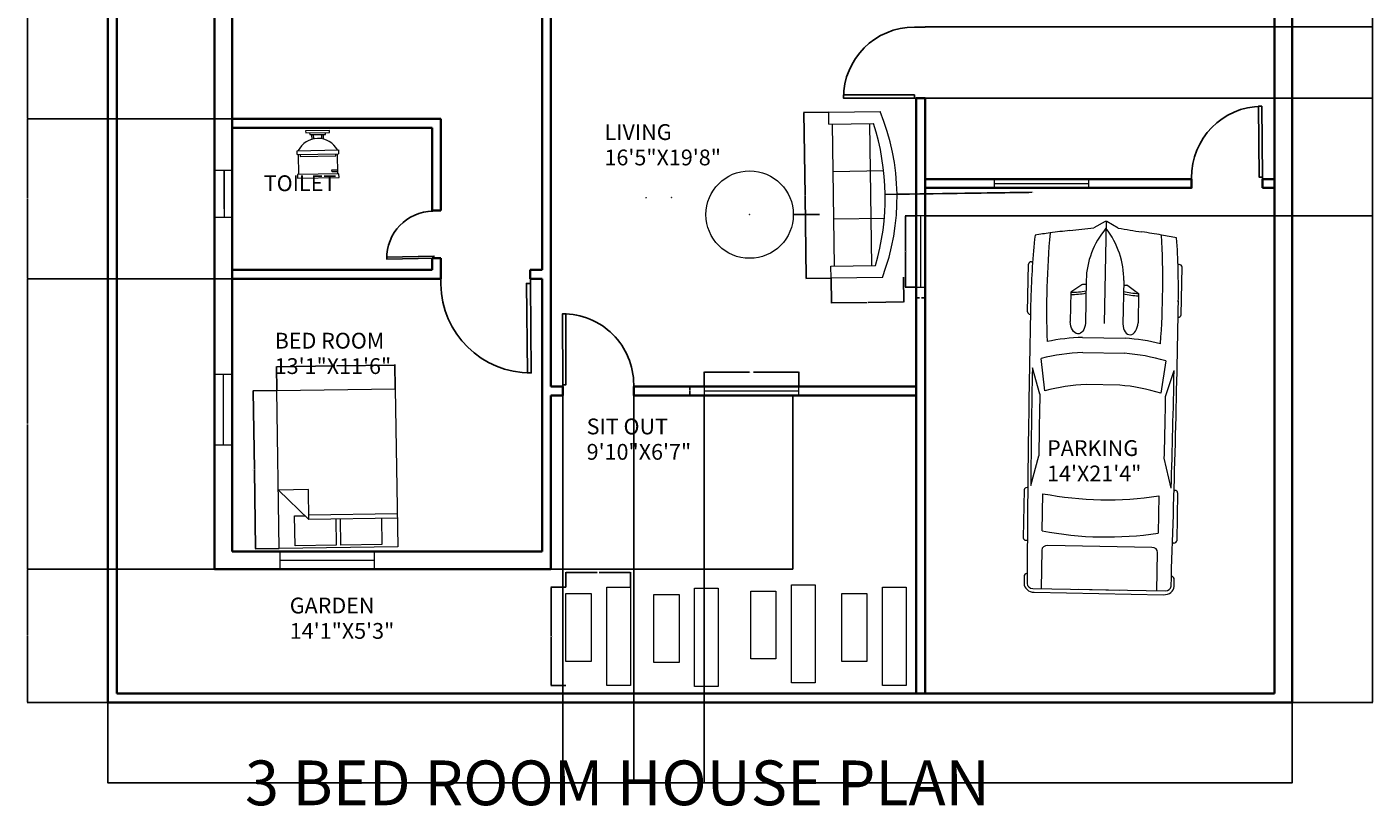
# Model space of a CAD drawing. Units: inches. Extents: x 267 to 949, y 280 to 1117.
# Tile 1 of 2: x 267 to 949, y 280 to 674. Entities that reach past the tile are written whole.
import ezdxf

# ---------------------------------------------------------------- set-up
doc = ezdxf.new("R2010")
doc.units = ezdxf.units.IN
for name, color, linetype, lineweight in [('A-ANNO-DIMS', 2, 'Continuous', 18), ('A-AREA-IDEN', 5, 'Continuous', 18), ('A-FLOR', 7, 'Continuous', 25), ('A-FLOR-FIXT', 3, 'Continuous', 18), ('C-PRKG-VEHI', 3, 'Continuous', 18), ('DOOR', 1, 'Continuous', 25), ('FUR', 3, 'Continuous', 18), ('L-HRDS-PVMT', 7, 'Continuous', 18), ('TEXT', 5, 'Continuous', 35), ('WALL', 7, 'Continuous', 35), ('WIN', 2, 'Continuous', 20)]:
    doc.layers.add(name, color=color, linetype=linetype, lineweight=lineweight)
doc.styles.get("Standard").update_dxf_attribs({"font": 'arial.ttf'})
doc.dimstyles.get("Standard").update_dxf_attribs({"dimtxt": 0.18, "dimasz": 0.18, "dimexe": 0.18, "dimexo": 0.0625, "dimgap": 0.09, "dimtad": 0, "dimtih": 1, "dimtoh": 1, "dimdec": 4, "dimzin": 0, "dimdsep": 46, "dimtxsty": 'Standard', "dimcen": 0.09, "dimadec": 0, "dimazin": 0, "dimtfac": 1, "dimtdec": 4, "dimtofl": 0, "dimtmove": 0, "dimatfit": 3, "dimfxl": 1, "dimtolj": 1, "dimtzin": 0, "dimarcsym": 0})

# ---------------------------------------------------------------- blocks, each defined once
blk = doc.blocks.new('*U5')
for p, q in [((0, 0), (0, -6)), ((40, 0), (40, -6))]:
    blk.add_line(p, q)
blk.add_lwpolyline([(0, 0), (0, 40), (1.75, 40), (1.75, 0)], close=True)
blk.add_arc((0, 0), 40, 0, 90)
blk = doc.blocks.new('*U6')
for p, q in [((-40, 0), (-40, 6)), ((0, 0), (0, 6))]:
    blk.add_line(p, q)
blk.add_lwpolyline([(0, 0), (0, -40), (-1.75, -40), (-1.75, 0)], close=True)
blk.add_arc((0, 0), 40, 180, 270)
blk = doc.blocks.new('*U4')
for p, q in [((0, 0), (0, 6)), ((40, 0), (40, 6))]:
    blk.add_line(p, q)
blk.add_lwpolyline([(0, 0), (0, -40), (1.75, -40), (1.75, 0)], close=True)
blk.add_arc((0, 0), 40, 270, 0)
blk = doc.blocks.new('*U2')
for p, q in [((0, 0), (0, -6)), ((40, 0), (40, -6))]:
    blk.add_line(p, q)
blk.add_lwpolyline([(0, 0), (0, 40), (1.75, 40), (1.75, 0)], close=True)
blk.add_arc((0, 0), 40, 0, 90)
blk = doc.blocks.new('Sofa - Roundback 7 ft.')
for p, q in [((-12.00002, -32.4421), (-12.00003, -6.5971)), ((11.99997, -32.4421), (11.99998, -6.5971)), ((-36.000027, -34), (-36.000027, -11.4696)), ((-35.999844, -13.3819), (35.9998, -13.3819)), ((35.99998, -34), (35.99998, -11.4696)), ((-36.000027, -32.4421), (35.99998, -32.4421))]:
    blk.add_line(p, q)
for points in [[(-36.000027, -34), (-42.000027, -34), (-42.000027, -8)], [(41.99998, -8), (41.99998, -34), (35.99998, -34)]]:
    blk.add_lwpolyline(points)
for centre, radius, start, end in [((0, -114.25), 114.25, 68.43141, 111.5686), ((-0.00001, -127.1968), 121.1968, 72.72033, 107.2797)]:
    blk.add_arc(centre, radius, start, end)
blk = doc.blocks.new('Bed - Queen')
for p, q in [((0, -80.00003), (0, 0)), ((0, 0), (59.99999, 0)), ((59.99999, 0), (59.99999, -80.00003)), ((7.99999, -1.2), (28.79998, -1.2)), ((7.99999, -14.4), (7.99999, -1.2)), ((28.79998, -1.2), (28.79998, -14.4)), ((31.19999, -1.2), (51.99999, -1.2)), ((31.19999, -14.4), (31.19999, -1.2)), ((51.99999, -1.2), (51.99999, -16.4)), ((0, -14.4), (44.8, -14.4)), ((44.8, -16.8), (0, -16.8)), ((59.99999, -29.6), (44.8, -14.4)), ((44.8, -14.4), (44.8, -29.6)), ((51.99999, -16.4), (46.79936, -16.4)), ((44.8, -29.6), (59.99999, -29.6)), ((59.99999, -80.00003), (0, -80.00003))]:
    blk.add_line(p, q)
blk = doc.blocks.new('*U11')
for p, q in [((21.1, 37.41), (21.1, 36.83)), ((46.55, 38.89), (22.35, 38.89)), ((47.8, 37.39), (47.8, 37.41)), ((87.99, 31.87), (74.76, 35.92)), ((134.31, 35.6), (119.29, 31.78)), ((135.45, 37.07), (135.45, 37.41)), ((136.7, 38.89), (160.9, 38.89)), ((162.15, 37.41), (162.15, 36.77)), ((70.03, 31.54), (86.41, 29.35)), ((138.42, 29.35), (157.25, 29.35)), ((186.47, 29.35), (167.01, 29.35)), ((186.47, -33.5), (186.47, 33.5)), ((188.4, -32.76), (188.4, 32.76)), ((164.52, 26.39), (164.52, -26.39)), ((32.27, 11.63), (36.13, 17.17)), ((36.13, 17.17), (50.94, 17.17)), ((29.77, 9.51), (51.68, 9.51)), ((32.12, 9.51), (32.12, 11.15)), ((58.92, -10.77), (58.92, 10.77)), ((66.55, -10.53), (66.55, 10.53)), ((82.74, 8.5), (82.74, -8.5)), ((186.47, -10.53), (186.47, 10.53)), ((3.27, 6.13), (0.1, 0.41)), ((0, 0), (51.68, 0)), ((0.1, -0.41), (3.27, -6.13)), ((29.77, -9.51), (51.68, -9.51)), ((32.12, -9.51), (32.12, -11.15)), ((32.27, -11.63), (36.13, -17.17)), ((36.13, -17.17), (50.94, -17.17)), ((86.41, -29.35), (70.03, -31.54)), ((87.99, -31.87), (74.76, -35.92)), ((134.31, -35.6), (119.29, -31.78)), ((157.25, -29.35), (138.42, -29.35)), ((167.01, -29.35), (186.47, -29.35)), ((21.1, -37.41), (21.1, -36.83)), ((46.55, -38.89), (22.35, -38.89)), ((47.8, -37.39), (47.8, -37.41)), ((135.45, -37.07), (135.45, -37.41)), ((136.7, -38.89), (160.9, -38.89)), ((162.15, -37.41), (162.15, -36.77))]:
    blk.add_line(p, q)
for centre, major_axis, ratio, start_param, end_param in [((266.03, -27.52), (0, 313.31), 0.842304, 1.367076, 1.39176), ((41.19, -490.86), (0, 528.23), 0.842304, 0.00281, 0.075598), ((22.35, 37.41), (0, -1.48), 0.842304, 3.141593, 4.712389), ((64.48, -10555.62), (0, 10593.03), 0.842304, -0.013397, 0.002797), ((46.55, 37.41), (0, 1.48), 0.842304, -1.570796, 0), ((64.48, -10555.62), (0, -10591.55), 0.842304, 3.133765, 3.140441), ((136.7, 37.41), (0, -1.48), 0.842304, 3.141593, 4.712389), ((160.9, 37.41), (0, 1.48), 0.842304, -1.570796, 0), ((180.63, 35.84), (0, 2.22), 0.842304, -0.013017, 1.249894), ((64.48, -10556.36), (0, 10595.31), 0.842304, -0.013397, -0.013017), ((183.98, 33.5), (0, -2.96), 0.842304, 1.570796, 3.128196), ((183.98, 32.76), (0, -5.25), 0.842304, 1.570796, 3.128196), ((259.18, -27.52), (0, -305.3), 0.842304, 4.528606, 4.561838), ((37.47, -593.96), (0, -623.33), 0.842304, 3.096046, 3.200911), ((134.4, 5.39), (0, -89.78), 0.842304, 4.449482, 4.652344), ((135.29, 5.39), (0, 81.77), 0.842304, 1.245306, 1.50788), ((149.6, 2.8), (0, -79.58), 0.842304, 4.372215, 4.640744), ((95.79, -3666.35), (0, -3698.24), 0.842304, 3.134049, 3.144098), ((17.08, 0), (0, 147.02), 0.842304, 4.511394, 4.913384), ((35.91, 0), (0, 147.02), 0.842304, 4.511394, 4.913384), ((167.01, 26.39), (0, 2.96), 0.842304, 0, 1.570796), ((-204.49, 52.4), (0, -250.96), 0.842304, 1.385369, 1.434372), ((13.04, 17.01), (0, 27.42), 0.842304, 4.435146, 4.718221), ((14.2, 17.01), (0, 27.42), 0.842304, 4.435146, 4.718221), ((50.79, 13.34), (6.34, -0.36), 0.603834, -1.395552, 1.581315), ((29.77, -46.66), (0, 56.17), 0.842304, 0, 0.590319), ((32.75, 11.15), (0, 0.74), 0.842304, 0.879714, 1.570796), ((0.62, 0), (0, -0.74), 0.842304, 4.131459, 5.293319), ((-204.49, -52.4), (0, 250.96), 0.842304, -1.434372, -1.385369), ((29.77, 46.66), (0, 56.17), 0.842304, 2.551274, 3.141593), ((32.75, -11.15), (0, -0.74), 0.842304, 4.712389, 5.403472), ((13.04, -17.01), (0, -27.42), 0.842304, 1.564964, 1.848039), ((14.2, -17.01), (0, -27.42), 0.842304, 1.564964, 1.848039), ((134.4, -5.39), (0, -89.78), 0.842304, -1.510751, -1.307889), ((135.29, -5.39), (0, -81.77), 0.842304, -1.50788, -1.245306), ((149.6, -2.8), (0, -79.58), 0.842304, -1.499151, -1.230623), ((259.18, 27.52), (0, 305.3), 0.842304, 1.721348, 1.754579), ((167.01, -26.39), (0, -2.96), 0.842304, 4.712389, 6.283185), ((266.03, 27.52), (0, 313.31), 0.842304, 1.749832, 1.774517), ((37.47, 593.96), (0, -623.33), 0.842304, -0.059319, 0.045547), ((95.79, 3666.35), (0, -3698.24), 0.842304, -0.002505, 0.007544), ((183.98, -33.5), (0, 2.96), 0.842304, 3.15499, 4.712389), ((183.98, -32.76), (0, -5.25), 0.842304, 0.013397, 1.570796), ((41.19, 490.86), (0, -528.23), 0.842304, -0.075598, -0.00281), ((22.35, -37.41), (0, 1.48), 0.842304, 1.570796, 3.141593), ((64.48, 10555.62), (0, 10593.03), 0.842304, 3.138796, 3.15499), ((46.55, -37.41), (0, -1.48), 0.842304, 0, 1.570796), ((64.48, 10555.62), (0, -10591.55), 0.842304, 0.001152, 0.007828), ((136.7, -37.41), (0, -1.48), 0.842304, -1.570796, 0), ((160.9, -37.41), (0, 1.48), 0.842304, 3.141593, 4.712389), ((180.63, -35.84), (0, -2.22), 0.842304, -1.249894, 0.013017), ((64.48, 10556.36), (0, 10595.31), 0.842304, 3.15461, 3.15499)]:
    blk.add_ellipse(centre, major_axis=major_axis, ratio=ratio, start_param=start_param, end_param=end_param)
at = {"extrusion": (0, 0, -1)}
blk.add_ellipse((50.79, -13.34), major_axis=(6.34, 0.36), ratio=0.603834, start_param=-1.395552, end_param=1.581315, dxfattribs=at)
blk = doc.blocks.new('*U13')
for p, q in [((-10, 22), (-10, 12)), ((-10, 21), (-7, 21)), ((-7, 21), (-7, 20)), ((10, 12), (10, 22)), ((-7, 20), (-10, 20)), ((10.5, 12), (-10.5, 12)), ((-10.5, 10), (-10.5, 12)), ((10.5, 10), (-10.5, 10)), ((9, 13), (-9, 13)), ((-9, 13), (-9, 12)), ((9, 12), (9, 13)), ((10.5, 12), (10.5, 10)), ((4, 2), (-4, 2)), ((-4, 2), (-4, 1)), ((-3, 4.4065), (-3, 2)), ((-2, 2), (-2, 4.1658)), ((2, 4.1658), (2, 2)), ((3, 2), (3, 4.4065)), ((4, 1), (4, 2))]:
    blk.add_line(p, q)
for points in [[(10.5, 22), (10.5, 24), (-10.5, 24), (-10.5, 22)], [(6, 0), (6, 1), (-6, 1), (-6, 0)]]:
    blk.add_lwpolyline(points, close=True)
blk.add_arc((0, 15.3333), 11.3333, 208.0725, 331.9275)
blk = doc.blocks.new('WIN-36x9')
for p, q in [((0, 36), (9, 36)), ((0, 0), (0, 36)), ((4.5, 36), (4.5, 0)), ((9, 36), (9, 0)), ((9, 0), (0, 0))]:
    blk.add_line(p, q)
blk = doc.blocks.new('WIN-48x4_5')
for p, q in [((0, 4.5), (0, 0)), ((48, 4.5), (0, 4.5)), ((0, 2.25), (48, 2.25)), ((48, 0), (48, 4.5)), ((0, 0), (48, 0))]:
    blk.add_line(p, q)
blk = doc.blocks.new('WIN-36x4_5')
for p, q in [((0, 4.5), (0, 0)), ((36, 4.5), (0, 4.5)), ((0, 2.25), (36, 2.25)), ((36, 0), (36, 4.5)), ((0, 0), (36, 0))]:
    blk.add_line(p, q)
blk = doc.blocks.new('PAVER-STAGGERED-PAIR')
for points in [[(20.7, 49.67), (32.65, 49.67), (32.65, 0), (20.7, 0)], [(0, 46.48), (12.8, 46.48), (12.8, 12.15), (0, 12.15)]]:
    blk.add_lwpolyline(points, close=True)
blk = doc.blocks.new('*D19')
at = {"layer": 'A-ANNO-DIMS', "color": 0, "lineweight": -2, "transparency": 16777216}
for p, q in [((539.76, 390.37), (532.19, 390.37)), ((532.37, 390.19), (532.37, 365.71)), ((532.37, 340.87), (532.37, 365.35)), ((539.76, 340.69), (532.19, 340.69))]:
    blk.add_line(p, q, dxfattribs=at)
at = {"layer": 'A-ANNO-DIMS', "color": 0, "transparency": 16777216}
for points in [[(532.34, 390.19), (532.4, 390.19), (532.37, 390.37)], [(532.34, 340.87), (532.4, 340.87), (532.37, 340.69)]]:
    blk.add_solid(points, dxfattribs=at)
at = {"layer": 'Defpoints', "color": 0, "transparency": 16777216}
for p in [(532.37, 390.37), (539.82, 390.37), (539.82, 340.69)]:
    blk.add_point(p, dxfattribs=at)
at = {"layer": 'A-ANNO-DIMS', "color": 0, "transparency": 16777216, "insert": (532.37, 365.53), "char_height": 0.18, "attachment_point": 5}
blk.add_mtext('\\A1;PAVERS 50 TYP.', dxfattribs=at)
blk = doc.blocks.new('*D20')
at = {"layer": 'A-ANNO-DIMS', "color": 0, "lineweight": -2, "transparency": 16777216}
for p, q in [((539.82, 390.43), (539.82, 398)), ((540, 397.82), (555.62, 397.82)), ((572.29, 397.82), (556.67, 397.82)), ((572.47, 390.43), (572.47, 398))]:
    blk.add_line(p, q, dxfattribs=at)
at = {"layer": 'A-ANNO-DIMS', "color": 0, "transparency": 16777216}
for points in [[(540, 397.85), (540, 397.79), (539.82, 397.82)], [(572.29, 397.85), (572.29, 397.79), (572.47, 397.82)]]:
    blk.add_solid(points, dxfattribs=at)
at = {"layer": 'Defpoints', "color": 0, "transparency": 16777216}
for p in [(572.47, 397.82), (539.82, 390.37), (572.47, 390.37)]:
    blk.add_point(p, dxfattribs=at)
at = {"layer": 'A-ANNO-DIMS', "color": 0, "transparency": 16777216, "insert": (556.15, 397.82), "char_height": 0.18, "attachment_point": 5}
blk.add_mtext('\\A1;33 TYP.', dxfattribs=at)
blk = doc.blocks.new('*D21')
at = {"layer": 'A-ANNO-DIMS', "color": 0, "lineweight": -2, "transparency": 16777216}
for p, q in [((393.3, 489.95), (381.19, 489.77)), ((381.37, 489.59), (381.98, 449.96)), ((382.59, 409.96), (381.98, 449.59)), ((394.53, 409.96), (382.42, 409.78))]:
    blk.add_line(p, q, dxfattribs=at)
at = {"layer": 'A-ANNO-DIMS', "color": 0, "transparency": 16777216}
for points in [[(381.4, 489.59), (381.34, 489.59), (381.37, 489.77)], [(382.62, 409.96), (382.56, 409.96), (382.6, 409.78)]]:
    blk.add_solid(points, dxfattribs=at)
at = {"layer": 'Defpoints', "color": 0, "transparency": 16777216}
for p in [(393.36, 489.95), (382.6, 409.78), (394.59, 409.96)]:
    blk.add_point(p, dxfattribs=at)
at = {"layer": 'A-ANNO-DIMS', "color": 0, "transparency": 16777216, "insert": (381.98, 449.77), "char_height": 0.18, "attachment_point": 5}
blk.add_mtext('\\A1;QUEEN BED 80 TYP.', dxfattribs=at)
blk = doc.blocks.new('*D22')
at = {"layer": 'A-ANNO-DIMS', "color": 0, "lineweight": -2, "transparency": 16777216}
for p, q in [((393.36, 490.02), (393.18, 502.13)), ((393.36, 501.96), (422.65, 502.41)), ((452.99, 502.87), (423.7, 502.42)), ((453.36, 490.94), (453.17, 503.06))]:
    blk.add_line(p, q, dxfattribs=at)
at = {"layer": 'A-ANNO-DIMS', "color": 0, "transparency": 16777216}
for points in [[(393.36, 501.99), (393.36, 501.93), (393.18, 501.95)], [(452.99, 502.9), (452.99, 502.84), (453.17, 502.88)]]:
    blk.add_solid(points, dxfattribs=at)
at = {"layer": 'Defpoints', "color": 0, "transparency": 16777216}
for p in [(393.18, 501.95), (393.36, 489.95), (453.36, 490.88)]:
    blk.add_point(p, dxfattribs=at)
at = {"layer": 'A-ANNO-DIMS', "color": 0, "transparency": 16777216, "insert": (423.18, 502.41), "char_height": 0.18, "attachment_point": 5}
blk.add_mtext('\\A1;60 TYP.', dxfattribs=at)
blk = doc.blocks.new('*D27')
at = {"layer": 'A-ANNO-DIMS', "color": 0, "lineweight": -2, "transparency": 16777216}
for p, q in [((717.18, 578.34), (711.66, 578.34)), ((711.84, 578.16), (711.84, 560.52)), ((711.84, 542.52), (711.84, 560.16)), ((717.18, 542.34), (711.66, 542.34))]:
    blk.add_line(p, q, dxfattribs=at)
at = {"layer": 'A-ANNO-DIMS', "color": 0, "transparency": 16777216}
for points in [[(711.81, 578.16), (711.87, 578.16), (711.84, 578.34)], [(711.81, 542.52), (711.87, 542.52), (711.84, 542.34)]]:
    blk.add_solid(points, dxfattribs=at)
at = {"layer": 'Defpoints', "color": 0, "transparency": 16777216}
for p in [(717.24, 578.34), (711.84, 542.34), (717.24, 542.34)]:
    blk.add_point(p, dxfattribs=at)
at = {"layer": 'A-ANNO-DIMS', "color": 0, "transparency": 16777216, "insert": (711.84, 560.34), "char_height": 0.18, "attachment_point": 5}
blk.add_mtext('\\A1;WIN. C 36 TYP.', dxfattribs=at)
blk = doc.blocks.new('*D28')
at = {"layer": 'A-ANNO-DIMS', "color": 0, "lineweight": -2, "transparency": 16777216}
for p, q in [((717.24, 542.28), (717.24, 536.76)), ((721.74, 542.28), (721.74, 536.76)), ((717.42, 536.94), (719.03, 536.94)), ((721.56, 536.94), (719.95, 536.94))]:
    blk.add_line(p, q, dxfattribs=at)
at = {"layer": 'A-ANNO-DIMS', "color": 0, "transparency": 16777216}
for points in [[(717.42, 536.97), (717.42, 536.91), (717.24, 536.94)], [(721.56, 536.97), (721.56, 536.91), (721.74, 536.94)]]:
    blk.add_solid(points, dxfattribs=at)
at = {"layer": 'Defpoints', "color": 0, "transparency": 16777216}
for p in [(717.24, 542.34), (721.74, 542.34), (721.74, 536.94)]:
    blk.add_point(p, dxfattribs=at)
at = {"layer": 'A-ANNO-DIMS', "color": 0, "transparency": 16777216, "insert": (719.49, 536.94), "char_height": 0.18, "attachment_point": 5}
blk.add_mtext('\\A1;5 TYP.', dxfattribs=at)
blk = doc.blocks.new('*D29')
at = {"layer": 'A-ANNO-DIMS', "color": 0, "lineweight": -2, "transparency": 16777216}
for p, q in [((609.82, 492.08), (609.82, 499.4)), ((610, 499.22), (632.84, 499.22)), ((657.64, 499.22), (634.79, 499.22)), ((657.82, 492.08), (657.82, 499.4))]:
    blk.add_line(p, q, dxfattribs=at)
at = {"layer": 'A-ANNO-DIMS', "color": 0, "transparency": 16777216}
for points in [[(610, 499.25), (610, 499.19), (609.82, 499.22)], [(657.64, 499.25), (657.64, 499.19), (657.82, 499.22)]]:
    blk.add_solid(points, dxfattribs=at)
at = {"layer": 'Defpoints', "color": 0, "transparency": 16777216}
for p in [(657.82, 499.22), (609.82, 492.02), (657.82, 492.02)]:
    blk.add_point(p, dxfattribs=at)
at = {"layer": 'A-ANNO-DIMS', "color": 0, "transparency": 16777216, "insert": (633.82, 499.22), "char_height": 0.18, "attachment_point": 5}
blk.add_mtext('\\A1;WIN. D 48 TYP.', dxfattribs=at)
blk = doc.blocks.new('*D30')
at = {"layer": 'A-ANNO-DIMS', "color": 0, "lineweight": -2, "transparency": 16777216}
for p, q in [((609.75, 492.02), (602.44, 492.02)), ((602.62, 491.84), (602.62, 489.95)), ((609.75, 487.52), (602.44, 487.52)), ((602.62, 487.7), (602.62, 489.59))]:
    blk.add_line(p, q, dxfattribs=at)
at = {"layer": 'A-ANNO-DIMS', "color": 0, "transparency": 16777216}
for points in [[(602.59, 491.84), (602.65, 491.84), (602.62, 492.02)], [(602.59, 487.7), (602.65, 487.7), (602.62, 487.52)]]:
    blk.add_solid(points, dxfattribs=at)
at = {"layer": 'Defpoints', "color": 0, "transparency": 16777216}
for p in [(602.62, 492.02), (609.82, 492.02), (609.82, 487.52)]:
    blk.add_point(p, dxfattribs=at)
at = {"layer": 'A-ANNO-DIMS', "color": 0, "transparency": 16777216, "insert": (602.62, 489.77), "char_height": 0.18, "attachment_point": 5}
blk.add_mtext('\\A1;5 TYP.', dxfattribs=at)
blk = doc.blocks.new('*D31')
at = {"layer": 'A-ANNO-DIMS', "color": 0, "lineweight": -2, "transparency": 16777216}
for p, q in [((672.92, 630.87), (660.21, 630.7)), ((660.39, 630.52), (660.97, 588.89)), ((661.56, 546.89), (660.98, 588.52)), ((674.1, 546.88), (661.39, 546.7))]:
    blk.add_line(p, q, dxfattribs=at)
at = {"layer": 'A-ANNO-DIMS', "color": 0, "transparency": 16777216}
for points in [[(660.42, 630.52), (660.36, 630.52), (660.39, 630.7)], [(661.59, 546.89), (661.53, 546.89), (661.57, 546.71)]]:
    blk.add_solid(points, dxfattribs=at)
at = {"layer": 'Defpoints', "color": 0, "transparency": 16777216}
for p in [(672.98, 630.88), (661.57, 546.71), (674.16, 546.88)]:
    blk.add_point(p, dxfattribs=at)
at = {"layer": 'A-ANNO-DIMS', "color": 0, "transparency": 16777216, "insert": (660.98, 588.7), "char_height": 0.18, "attachment_point": 5}
blk.add_mtext('\\A1;SOFA 84', dxfattribs=at)
blk = doc.blocks.new('*D32')
at = {"layer": 'A-ANNO-DIMS', "color": 0, "lineweight": -2, "transparency": 16777216}
for p, q in [((674.16, 546.82), (674.34, 534.11)), ((710.83, 547.34), (711.01, 534.62)), ((674.52, 534.29), (692.45, 534.54)), ((710.82, 534.8), (692.89, 534.55))]:
    blk.add_line(p, q, dxfattribs=at)
at = {"layer": 'A-ANNO-DIMS', "color": 0, "transparency": 16777216}
for points in [[(674.52, 534.32), (674.52, 534.26), (674.34, 534.29)], [(710.82, 534.83), (710.82, 534.77), (711, 534.8)]]:
    blk.add_solid(points, dxfattribs=at)
at = {"layer": 'Defpoints', "color": 0, "transparency": 16777216}
for p in [(674.16, 546.88), (710.83, 547.4), (711, 534.8)]:
    blk.add_point(p, dxfattribs=at)
at = {"layer": 'A-ANNO-DIMS', "color": 0, "transparency": 16777216, "insert": (692.67, 534.54), "char_height": 0.18, "attachment_point": 5}
blk.add_mtext('\\A1;37', dxfattribs=at)
blk = doc.blocks.new('*D35')
at = {"layer": 'A-ANNO-DIMS', "color": 0, "lineweight": -2, "transparency": 16777216}
for p, q in [((307.74, 331.96), (307.74, 291.14)), ((907.74, 331.96), (907.74, 291.14)), ((307.92, 291.32), (607.45, 291.32)), ((907.56, 291.32), (608.03, 291.32))]:
    blk.add_line(p, q, dxfattribs=at)
at = {"layer": 'A-ANNO-DIMS', "color": 0, "transparency": 16777216}
for points in [[(307.92, 291.35), (307.92, 291.29), (307.74, 291.32)], [(907.56, 291.35), (907.56, 291.29), (907.74, 291.32)]]:
    blk.add_solid(points, dxfattribs=at)
at = {"layer": 'Defpoints', "color": 0, "transparency": 16777216}
for p in [(307.74, 332.02), (907.74, 332.02), (907.74, 291.32)]:
    blk.add_point(p, dxfattribs=at)
at = {"layer": 'A-ANNO-DIMS', "color": 0, "transparency": 16777216, "insert": (607.74, 291.32), "char_height": 0.18, "attachment_point": 5}
blk.add_mtext('\\A1;600', dxfattribs=at)
blk = doc.blocks.new('*D36')
at = {"layer": 'A-ANNO-DIMS', "color": 0, "lineweight": -2, "transparency": 16777216}
for p, q in [((907.8, 1052.02), (948.62, 1052.02)), ((948.44, 1051.84), (948.44, 692.2)), ((948.44, 332.2), (948.44, 691.84)), ((907.8, 332.02), (948.62, 332.02))]:
    blk.add_line(p, q, dxfattribs=at)
at = {"layer": 'A-ANNO-DIMS', "color": 0, "transparency": 16777216}
for points in [[(948.41, 1051.84), (948.47, 1051.84), (948.44, 1052.02)], [(948.41, 332.2), (948.47, 332.2), (948.44, 332.02)]]:
    blk.add_solid(points, dxfattribs=at)
at = {"layer": 'Defpoints', "color": 0, "transparency": 16777216}
for p in [(907.74, 1052.02), (948.44, 1052.02), (907.74, 332.02)]:
    blk.add_point(p, dxfattribs=at)
at = {"layer": 'A-ANNO-DIMS', "color": 0, "transparency": 16777216, "insert": (948.44, 692.02), "char_height": 0.18, "attachment_point": 5}
blk.add_mtext('\\A1;720', dxfattribs=at)
blk = doc.blocks.new('*D41')
at = {"layer": 'A-ANNO-DIMS', "color": 0, "lineweight": -2, "transparency": 16777216}
for p, q in [((361.68, 399.52), (266.86, 399.52)), ((267.04, 399.34), (267.04, 365.95)), ((267.04, 332.2), (267.04, 365.59)), ((307.68, 332.02), (266.86, 332.02))]:
    blk.add_line(p, q, dxfattribs=at)
at = {"layer": 'A-ANNO-DIMS', "color": 0, "transparency": 16777216}
for points in [[(267.01, 399.34), (267.07, 399.34), (267.04, 399.52)], [(267.01, 332.2), (267.07, 332.2), (267.04, 332.02)]]:
    blk.add_solid(points, dxfattribs=at)
at = {"layer": 'Defpoints', "color": 0, "transparency": 16777216}
for p in [(267.04, 399.52), (361.74, 399.52), (307.74, 332.02)]:
    blk.add_point(p, dxfattribs=at)
at = {"layer": 'A-ANNO-DIMS', "color": 0, "transparency": 16777216, "insert": (267.04, 365.77), "char_height": 0.18, "attachment_point": 5}
blk.add_mtext('\\A1;67.5', dxfattribs=at)
blk = doc.blocks.new('*D42')
at = {"layer": 'A-ANNO-DIMS', "color": 0, "lineweight": -2, "transparency": 16777216}
for p, q in [((370.68, 546.52), (266.86, 546.52)), ((267.04, 546.34), (267.04, 473.2)), ((267.04, 399.7), (267.04, 472.84)), ((361.68, 399.52), (266.86, 399.52))]:
    blk.add_line(p, q, dxfattribs=at)
at = {"layer": 'A-ANNO-DIMS', "color": 0, "transparency": 16777216}
for points in [[(267.01, 546.34), (267.07, 546.34), (267.04, 546.52)], [(267.01, 399.7), (267.07, 399.7), (267.04, 399.52)]]:
    blk.add_solid(points, dxfattribs=at)
at = {"layer": 'Defpoints', "color": 0, "transparency": 16777216}
for p in [(267.04, 546.52), (370.74, 546.52), (361.74, 399.52)]:
    blk.add_point(p, dxfattribs=at)
at = {"layer": 'A-ANNO-DIMS', "color": 0, "transparency": 16777216, "insert": (267.04, 473.02), "char_height": 0.18, "attachment_point": 5}
blk.add_mtext('\\A1;147', dxfattribs=at)
blk = doc.blocks.new('*D43')
at = {"layer": 'A-ANNO-DIMS', "color": 0, "lineweight": -2, "transparency": 16777216}
for p, q in [((370.68, 627.52), (266.86, 627.52)), ((267.04, 627.34), (267.04, 587.2)), ((267.04, 546.7), (267.04, 586.84)), ((370.68, 546.52), (266.86, 546.52))]:
    blk.add_line(p, q, dxfattribs=at)
at = {"layer": 'A-ANNO-DIMS', "color": 0, "transparency": 16777216}
for points in [[(267.01, 627.34), (267.07, 627.34), (267.04, 627.52)], [(267.01, 546.7), (267.07, 546.7), (267.04, 546.52)]]:
    blk.add_solid(points, dxfattribs=at)
at = {"layer": 'Defpoints', "color": 0, "transparency": 16777216}
for p in [(267.04, 627.52), (370.74, 627.52), (370.74, 546.52)]:
    blk.add_point(p, dxfattribs=at)
at = {"layer": 'A-ANNO-DIMS', "color": 0, "transparency": 16777216, "insert": (267.04, 587.02), "char_height": 0.18, "attachment_point": 5}
blk.add_mtext('\\A1;81', dxfattribs=at)
blk = doc.blocks.new('*D44')
at = {"layer": 'A-ANNO-DIMS', "color": 0, "lineweight": -2, "transparency": 16777216}
for p, q in [((370.68, 822.02), (266.86, 822.02)), ((267.04, 821.84), (267.04, 724.95)), ((267.04, 627.7), (267.04, 724.59)), ((370.68, 627.52), (266.86, 627.52))]:
    blk.add_line(p, q, dxfattribs=at)
at = {"layer": 'A-ANNO-DIMS', "color": 0, "transparency": 16777216}
for points in [[(267.01, 821.84), (267.07, 821.84), (267.04, 822.02)], [(267.01, 627.7), (267.07, 627.7), (267.04, 627.52)]]:
    blk.add_solid(points, dxfattribs=at)
at = {"layer": 'Defpoints', "color": 0, "transparency": 16777216}
for p in [(267.04, 822.02), (370.74, 822.02), (370.74, 627.52)]:
    blk.add_point(p, dxfattribs=at)
at = {"layer": 'A-ANNO-DIMS', "color": 0, "transparency": 16777216, "insert": (267.04, 724.77), "char_height": 0.18, "attachment_point": 5}
blk.add_mtext('\\A1;194.5', dxfattribs=at)
blk = doc.blocks.new('*D47')
at = {"layer": 'A-ANNO-DIMS', "color": 0, "lineweight": -2, "transparency": 16777216}
for p, q in [((538.24, 487.46), (538.24, 291.14)), ((574.24, 487.46), (574.24, 291.14)), ((538.42, 291.32), (556.02, 291.32)), ((574.06, 291.32), (556.46, 291.32))]:
    blk.add_line(p, q, dxfattribs=at)
at = {"layer": 'A-ANNO-DIMS', "color": 0, "transparency": 16777216}
for points in [[(538.42, 291.35), (538.42, 291.29), (538.24, 291.32)], [(574.06, 291.35), (574.06, 291.29), (574.24, 291.32)]]:
    blk.add_solid(points, dxfattribs=at)
at = {"layer": 'Defpoints', "color": 0, "transparency": 16777216}
for p in [(538.24, 487.52), (574.24, 487.52), (574.24, 291.32)]:
    blk.add_point(p, dxfattribs=at)
at = {"layer": 'A-ANNO-DIMS', "color": 0, "transparency": 16777216, "insert": (556.24, 291.32), "char_height": 0.18, "attachment_point": 5}
blk.add_mtext('\\A1;36', dxfattribs=at)
blk = doc.blocks.new('*D48')
at = {"layer": 'A-ANNO-DIMS', "color": 0, "lineweight": -2, "transparency": 16777216}
for p, q in [((574.24, 487.46), (574.24, 291.14)), ((609.82, 487.46), (609.82, 291.14)), ((574.42, 291.32), (591.56, 291.32)), ((609.64, 291.32), (592.49, 291.32))]:
    blk.add_line(p, q, dxfattribs=at)
at = {"layer": 'A-ANNO-DIMS', "color": 0, "transparency": 16777216}
for points in [[(574.42, 291.35), (574.42, 291.29), (574.24, 291.32)], [(609.64, 291.35), (609.64, 291.29), (609.82, 291.32)]]:
    blk.add_solid(points, dxfattribs=at)
at = {"layer": 'Defpoints', "color": 0, "transparency": 16777216}
for p in [(574.24, 487.52), (609.82, 487.52), (609.82, 291.32)]:
    blk.add_point(p, dxfattribs=at)
at = {"layer": 'A-ANNO-DIMS', "color": 0, "transparency": 16777216, "insert": (592.03, 291.32), "char_height": 0.18, "attachment_point": 5}
blk.add_mtext('\\A1;35.575', dxfattribs=at)
blk = doc.blocks.new('*D49')
at = {"layer": 'A-ANNO-DIMS', "color": 0, "lineweight": -2, "transparency": 16777216}
for p, q in [((721.8, 674.02), (948.62, 674.02)), ((948.44, 673.84), (948.44, 656.2)), ((948.44, 638.2), (948.44, 655.84)), ((721.8, 638.02), (948.62, 638.02))]:
    blk.add_line(p, q, dxfattribs=at)
at = {"layer": 'A-ANNO-DIMS', "color": 0, "transparency": 16777216}
for points in [[(948.41, 673.84), (948.47, 673.84), (948.44, 674.02)], [(948.41, 638.2), (948.47, 638.2), (948.44, 638.02)]]:
    blk.add_solid(points, dxfattribs=at)
at = {"layer": 'Defpoints', "color": 0, "transparency": 16777216}
for p in [(721.74, 674.02), (948.44, 674.02), (721.74, 638.02)]:
    blk.add_point(p, dxfattribs=at)
at = {"layer": 'A-ANNO-DIMS', "color": 0, "transparency": 16777216, "insert": (948.44, 656.02), "char_height": 0.18, "attachment_point": 5}
blk.add_mtext('\\A1;36', dxfattribs=at)
blk = doc.blocks.new('*D50')
at = {"layer": 'A-ANNO-DIMS', "color": 0, "lineweight": -2, "transparency": 16777216}
for p, q in [((721.8, 638.02), (948.62, 638.02)), ((948.44, 637.84), (948.44, 608.36)), ((948.44, 578.52), (948.44, 608)), ((721.8, 578.34), (948.62, 578.34))]:
    blk.add_line(p, q, dxfattribs=at)
at = {"layer": 'A-ANNO-DIMS', "color": 0, "transparency": 16777216}
for points in [[(948.41, 637.84), (948.47, 637.84), (948.44, 638.02)], [(948.41, 578.52), (948.47, 578.52), (948.44, 578.34)]]:
    blk.add_solid(points, dxfattribs=at)
at = {"layer": 'Defpoints', "color": 0, "transparency": 16777216}
for p in [(721.74, 638.02), (948.44, 638.02), (721.74, 578.34)]:
    blk.add_point(p, dxfattribs=at)
at = {"layer": 'A-ANNO-DIMS', "color": 0, "transparency": 16777216, "insert": (948.44, 608.18), "char_height": 0.18, "attachment_point": 5}
blk.add_mtext('\\A1;59.68', dxfattribs=at)
blk = doc.blocks.new('*D51')
at = {"layer": 'A-ANNO-DIMS', "color": 0, "lineweight": -2, "transparency": 16777216}
for p, q in [((632.79, 579.02), (632.97, 579.02)), ((632.88, 578.93), (632.88, 579.11)), ((668.3, 579.02), (655.2, 579.02))]:
    blk.add_line(p, q, dxfattribs=at)
at = {"layer": 'A-ANNO-DIMS', "color": 0, "transparency": 16777216}
blk.add_solid([(655.2, 579.05), (655.2, 578.99), (655.02, 579.02)], dxfattribs=at)
at = {"layer": 'Defpoints', "color": 0, "transparency": 16777216}
for p in [(610.75, 579.02), (655.02, 579.02)]:
    blk.add_point(p, dxfattribs=at)
at = {"layer": 'A-ANNO-DIMS', "color": 0, "transparency": 16777216, "insert": (668.8, 579.02), "char_height": 0.18, "attachment_point": 5}
blk.add_mtext('\\A1;∅44.27', dxfattribs=at)
blk = doc.blocks.new('*D52')
at = {"layer": 'A-ANNO-DIMS', "color": 0, "lineweight": -2, "transparency": 16777216}
for p, q in [((580.3, 587.57), (580.48, 587.57)), ((580.39, 587.48), (580.39, 587.66)), ((774.28, 590.29), (701.75, 589.28))]:
    blk.add_line(p, q, dxfattribs=at)
at = {"layer": 'A-ANNO-DIMS', "color": 0, "transparency": 16777216}
blk.add_solid([(701.75, 589.31), (701.75, 589.25), (701.57, 589.27)], dxfattribs=at)
at = {"layer": 'Defpoints', "color": 0, "transparency": 16777216}
for p in [(580.39, 587.57), (701.57, 589.27)]:
    blk.add_point(p, dxfattribs=at)
at = {"layer": 'A-ANNO-DIMS', "color": 0, "transparency": 16777216, "insert": (774.76, 590.29), "char_height": 0.18, "attachment_point": 5}
blk.add_mtext('\\A1;R121.2', dxfattribs=at)
blk = doc.blocks.new('*D53')
at = {"layer": 'A-ANNO-DIMS', "color": 0, "lineweight": -2, "transparency": 16777216}
for p, q in [((593.24, 587.75), (593.42, 587.75)), ((593.33, 587.66), (593.33, 587.84)), ((776.11, 590.32), (707.75, 589.36))]:
    blk.add_line(p, q, dxfattribs=at)
at = {"layer": 'A-ANNO-DIMS', "color": 0, "transparency": 16777216}
blk.add_solid([(707.75, 589.39), (707.75, 589.33), (707.57, 589.36)], dxfattribs=at)
at = {"layer": 'Defpoints', "color": 0, "transparency": 16777216}
for p in [(593.33, 587.75), (707.57, 589.36)]:
    blk.add_point(p, dxfattribs=at)
at = {"layer": 'A-ANNO-DIMS', "color": 0, "transparency": 16777216, "insert": (776.66, 590.32), "char_height": 0.18, "attachment_point": 5}
blk.add_mtext('\\A1;R114.25', dxfattribs=at)

msp = doc.modelspace()

# ---------------------------------------------------------------- linework, layer by layer
at = {"layer": 'A-FLOR'}
for p in [(654.7409, 487.5219), (532.2409, 399.5219)]:
    msp.add_line(p, (654.7409, 399.5219), dxfattribs=at)
at = {"layer": 'FUR'}
msp.add_circle((632.8845, 579.0219), 22.1371, dxfattribs=at)
at = {"layer": 'WALL'}
for p, q in [((307.7409, 1052.0219), (307.7409, 332.0219)), ((907.7409, 1052.0219), (907.7409, 332.0219)), ((312.2409, 1043.0219), (312.2409, 336.5219)), ((361.7409, 1043.0219), (361.7409, 399.5219)), ((361.7409, 1043.0219), (361.7409, 399.5219)), ((361.7409, 1043.0219), (361.7409, 399.5219)), ((370.7409, 1043.0219), (370.7409, 408.5219)), ((898.7409, 1043.0219), (898.7409, 336.5219)), ((527.7409, 832.5219), (527.7409, 551.0219)), ((532.2409, 832.5219), (532.2409, 492.0219)), ((717.2409, 638.0219), (721.7409, 638.0219)), ((717.2409, 638.0219), (717.2409, 336.5219)), ((721.7409, 638.0219), (721.7409, 336.5219)), ((370.7409, 627.5219), (476.4951, 627.5219)), ((476.4951, 627.5219), (476.4951, 581.0219)), ((370.7409, 623.0219), (471.9951, 623.0219)), ((471.9951, 623.0219), (471.9951, 581.0219)), ((721.7409, 597.0219), (856.7409, 597.0219)), ((856.7409, 597.0219), (856.7409, 592.5219)), ((898.7409, 597.0219), (892.7409, 597.0219)), ((892.7409, 597.0219), (892.7409, 592.5219)), ((892.7409, 597.0219), (898.7409, 597.0219)), ((721.7409, 592.5219), (856.7409, 592.5219)), ((892.7409, 592.5219), (898.7409, 592.5219)), ((476.4951, 581.0219), (471.9951, 581.0219)), ((476.4951, 557.0219), (471.9951, 557.0219)), ((471.9951, 557.0219), (471.9951, 551.0219)), ((476.4951, 551.0219), (476.4951, 557.0219)), ((476.4951, 557.0219), (476.4951, 546.5219)), ((370.7409, 551.0219), (471.9951, 551.0219)), ((370.7409, 546.5219), (476.4951, 546.5219)), ((521.7409, 551.0219), (527.7409, 551.0219)), ((527.7409, 551.0219), (521.7409, 551.0219)), ((521.7409, 551.0219), (521.7409, 546.5219)), ((521.7409, 546.5219), (527.7409, 546.5219)), ((527.7409, 546.5219), (527.7409, 408.5219)), ((532.2409, 492.0219), (538.2409, 492.0219)), ((532.2409, 492.0219), (538.2409, 492.0219)), ((538.2409, 492.0219), (538.2409, 487.5219)), ((574.2409, 492.0219), (574.2409, 487.5219)), ((574.2409, 492.0219), (717.2409, 492.0219)), ((532.2409, 487.5219), (538.2409, 487.5219)), ((532.2409, 487.5219), (532.2409, 399.5219)), ((574.2409, 487.5219), (717.2409, 487.5219)), ((370.7409, 408.5219), (527.7409, 408.5219)), ((361.7409, 399.5219), (532.2409, 399.5219)), ((312.2409, 336.5219), (898.7409, 336.5219)), ((307.7409, 332.0219), (907.7409, 332.0219))]:
    msp.add_line(p, q, dxfattribs=at)
msp.add_lwpolyline([(605.4909, 336.5219), (593.5423, 336.5219)], dxfattribs=at)
at = {"layer": 'WIN'}
for p, q in [((361.7409, 601.5446), (370.7409, 601.5446)), ((361.7409, 577.5446), (361.7409, 601.5446)), ((366.6437, 581.9766), (366.6437, 601.5446)), ((366.6437, 601.5446), (366.6437, 577.5446)), ((370.7409, 601.5446), (370.7409, 577.5446)), ((370.7409, 577.5446), (361.7409, 577.5446)), ((394.8327, 408.5219), (394.8327, 399.5219)), ((442.8327, 408.5219), (394.8327, 408.5219)), ((394.8327, 404.0219), (442.8327, 404.0219)), ((442.8327, 399.5219), (442.8327, 408.5219)), ((394.8327, 399.5219), (442.8327, 399.5219))]:
    msp.add_line(p, q, dxfattribs=at)

# ---------------------------------------------------------------- block references
at = {"layer": 'A-FLOR-FIXT', "rotation": 180.9809891052875}
msp.add_blockref('*U13', (413.955, 621.5598), dxfattribs=at)
at = {"layer": 'C-PRKG-VEHI', "rotation": 268.8910973424977}
msp.add_blockref('*U11', (813.4923, 575.5556), dxfattribs=at)
at = {"layer": 'DOOR'}
for name, p, xscale, yscale, zscale, rotation in [('*U2', (716.3527, 638.0219), 0.898029023570897, 0.898029023570897, 0.898029023570897, 90), ('*U4', (892.6876, 597.9152), 0.89893798740989, 0.89893798740989, 0.89893798740989, 180.5661466738159), ('*U6', (472.9125, 556.9511), 0.5972278222085774, 0.5972278222085774, 0.5972278222085774, 271.1322933476318), ('*U5', (521.808, 544.2242), 1.133004395887791, 1.133004395887791, 1.133004395887791, 180.5661466738159), ('*U2', (538.2294, 492.91), 0.898029023570897, 0.898029023570897, 0.898029023570897, 0.1220590888270939)]:
    msp.add_blockref(name, p, dxfattribs=dict(at, xscale=xscale, yscale=yscale, zscale=zscale, rotation=rotation))
at = {"layer": 'FUR'}
for name, p, rotation in [('Sofa - Roundback 7 ft.', (707.5708, 589.3571), 270.8045766995283), ('Bed - Queen', (454.5871, 410.8862), 180.8809648164193)]:
    msp.add_blockref(name, p, dxfattribs=dict(at, rotation=rotation))
at = {"layer": 'L-HRDS-PVMT'}
for p in [(539.8225, 340.692), (584.3039, 340.197), (633.4412, 341.9018), (679.538, 340.692)]:
    msp.add_blockref('PAVER-STAGGERED-PAIR', p, dxfattribs=at)
at = {"layer": 'WIN'}
for name, p in [('WIN-48x4_5', (756.7187, 592.522)), ('WIN-36x9', (361.741, 462.2939)), ('WIN-48x4_5', (609.816, 487.522))]:
    msp.add_blockref(name, p, dxfattribs=at)
at = {"layer": 'WIN', "rotation": 269.9999999999998}
msp.add_blockref('WIN-36x4_5', (717.241, 578.3415), dxfattribs=at)

# ---------------------------------------------------------------- texts
at = {"layer": 'A-AREA-IDEN'}
for s, p in [('LIVING', (559.3484, 616.7953)), ('16\'5"X19\'8"', (559.3484, 603.944)), ('TOILET', (386.7314, 590.8926)), ('BED ROOM', (392.2623, 511.1825)), ('13\'1"X11\'6"', (392.2623, 498.3312)), ('SIT OUT', (550.314, 467.7654)), ('PARKING', (783.5808, 456.8223)), ('9\'10"X6\'7"', (550.314, 454.9141)), ('14\'X21\'4"', (783.5808, 443.971)), ('GARDEN', (399.9023, 377.1143)), ('14\'1"X5\'3"', (399.9023, 364.263))]:
    msp.add_text(s, height=8, dxfattribs=at).set_placement(p)
at = {"layer": 'TEXT'}
msp.add_text('3 BED ROOM HOUSE PLAN', height=22.670217, dxfattribs=at).set_placement((377.2654, 279.9988))

# ---------------------------------------------------------------- dimensions: what is measured, and where the dimension line sits
at = {"layer": 'A-ANNO-DIMS'}
for base, p1, p2, angle, override, picture, middle in [((948.4409, 1052.0219), (907.7409, 332.0219), (907.7409, 1052.0219), 90, {"dimdec": 0, "dimlfac": 1, "dimrnd": 0, "dimzin": 0, "dimdsep": 46, "dimlunit": 2}, '*D36', (948.4409, 692.0219)), ((267.0409, 822.0219), (370.7409, 627.5219), (370.7409, 822.0219), 90, {"dimdec": 1, "dimlfac": 1, "dimrnd": 0, "dimzin": 0, "dimdsep": 46, "dimlunit": 2}, '*D44', (267.0409, 724.7719)), ((948.4409, 674.0219), (721.7409, 638.0219), (721.7409, 674.0219), 90, {"dimdec": 0, "dimlfac": 1, "dimrnd": 0, "dimzin": 0, "dimdsep": 46, "dimlunit": 2}, '*D49', (948.4409, 656.0219)), ((948.4409, 638.0219), (721.7409, 578.3418), (721.7409, 638.0219), 90, {"dimdec": 2, "dimlfac": 1, "dimrnd": 0, "dimzin": 0, "dimdsep": 46, "dimlunit": 2}, '*D50', (948.4409, 608.1818)), ((267.0409, 627.5219), (370.7409, 546.5219), (370.7409, 627.5219), 90, {"dimdec": 0, "dimlfac": 1, "dimrnd": 0, "dimzin": 0, "dimdsep": 46, "dimlunit": 2}, '*D43', (267.0409, 587.0219)), ((267.0409, 546.5219), (361.7409, 399.5219), (370.7409, 546.5219), 90, {"dimdec": 0, "dimlfac": 1, "dimrnd": 0, "dimzin": 0, "dimdsep": 46, "dimlunit": 2}, '*D42', (267.0409, 473.0219)), ((711.0039, 534.7999), (674.1639, 546.8838), (710.8269, 547.3987), 0.8045767, {"dimdec": 0, "dimlfac": 1, "dimrnd": 0, "dimzin": 0, "dimdsep": 46, "dimlunit": 2}, '*D32', (692.6723, 534.5425)), ((267.0409, 399.5219), (307.7409, 332.0219), (361.7409, 399.5219), 90, {"dimdec": 1, "dimlfac": 1, "dimrnd": 0, "dimzin": 0, "dimdsep": 46, "dimlunit": 2}, '*D41', (267.0409, 365.7719))]:
    dim = msp.add_linear_dim(base=base, p1=p1, p2=p2, angle=angle, dimstyle='Standard', override=override, dxfattribs=at)
    dim.commit()
    dim.dimension.update_dxf_attribs({"geometry": picture, "text_midpoint": middle})
for base, p1, p2, angle, text, picture, middle in [((661.5651, 546.7069), (672.9844, 630.8755), (674.1639, 546.8838), 270.8045767, 'SOFA <>', '*D31', (660.9754, 588.7027)), ((711.8409, 542.3418), (717.2409, 578.3418), (717.2409, 542.3418), 270, 'WIN. C <> TYP.', '*D27', (711.8409, 560.3418)), ((393.1797, 501.9529), (453.3571, 490.8768), (393.3642, 489.9543), 180.8809648, '<> TYP.', '*D22', (423.1761, 502.4142)), ((602.6156731551, 492.0218814908), (609.8156731551, 487.5218814908), (609.8156731551, 492.0218814908), 90, '<> TYP.', '*D30', (602.6156731551, 489.7718814908)), ((382.5956, 409.7792), (393.3642, 489.9543), (394.5942, 409.9637), 270.8809648, 'QUEEN BED <> TYP.', '*D21', (381.9806, 449.7745)), ((532.3715, 390.3665), (539.8226, 340.6923), (539.8226, 390.3665), 90, 'PAVERS <> TYP.', '*D19', (532.3715, 365.5294))]:
    dim = msp.add_linear_dim(base=base, p1=p1, p2=p2, angle=angle, text=text, dimstyle='Standard', override={"dimdec": 0, "dimlfac": 1, "dimrnd": 0, "dimzin": 0, "dimdsep": 46, "dimlunit": 2}, dxfattribs=at)
    dim.commit()
    dim.dimension.update_dxf_attribs({"geometry": picture, "text_midpoint": middle})
for center, mpoint, override, picture, middle in [((580.3865, 587.571), (701.5714, 589.273), {"dimdec": 1, "dimlfac": 1, "dimrnd": 0, "dimzin": 0, "dimdsep": 46, "dimlunit": 2}, '*D52', (774.2823, 590.2942)), ((593.332, 587.7528), (707.5708, 589.357), {"dimdec": 2, "dimlfac": 1, "dimrnd": 0, "dimzin": 0, "dimdsep": 46, "dimlunit": 2}, '*D53', (776.114, 590.3195))]:
    dim = msp.add_radius_dim(center=center, mpoint=mpoint, dimstyle='Standard', override=override, dxfattribs=at)
    dim.commit()
    dim.dimension.update_dxf_attribs({"geometry": picture, "text_midpoint": middle, "dimtype": 164})
dim = msp.add_diameter_dim_2p(p1=(610.7473, 579.0219), p2=(655.0216, 579.022), dimstyle='Standard', override={"dimdec": 2, "dimlfac": 1, "dimrnd": 0, "dimzin": 0, "dimdsep": 46, "dimlunit": 2}, dxfattribs=at)
dim.commit()
dim.dimension.update_dxf_attribs({"geometry": '*D51', "text_midpoint": (668.3039, 579.022), "dimtype": 163})
for base, p1, p2, text, picture, middle in [((721.7408789529, 536.9418128038), (717.2408789529, 542.3418128038), (721.7408789529, 542.3418128038), '<> TYP.', '*D28', (719.4908789529, 536.9418128038)), ((657.8157, 499.2219), (609.8157, 492.0219), (657.8157, 492.0219), 'WIN. D <> TYP.', '*D29', (633.8157, 499.2219)), ((572.4677, 397.8176), (539.8226, 390.3665), (572.4677, 390.3665), '<> TYP.', '*D20', (556.1452, 397.8176))]:
    dim = msp.add_linear_dim(base=base, p1=p1, p2=p2, text=text, dimstyle='Standard', override={"dimdec": 0, "dimlfac": 1, "dimrnd": 0, "dimzin": 0, "dimdsep": 46, "dimlunit": 2}, dxfattribs=at)
    dim.commit()
    dim.dimension.update_dxf_attribs({"geometry": picture, "text_midpoint": middle})
for base, p1, p2, override, picture, middle in [((574.2409, 291.3219), (538.2409, 487.5219), (574.2409, 487.5219), {"dimdec": 0, "dimlfac": 1, "dimrnd": 0, "dimzin": 0, "dimdsep": 46, "dimlunit": 2}, '*D47', (556.2409, 291.3219)), ((609.8157, 291.3219), (574.2409, 487.5219), (609.8157, 487.5219), {"dimdec": 3, "dimlfac": 1, "dimrnd": 0, "dimzin": 0, "dimdsep": 46, "dimlunit": 2}, '*D48', (592.0283, 291.3219)), ((907.7409, 291.3219), (307.7409, 332.0219), (907.7409, 332.0219), {"dimdec": 0, "dimlfac": 1, "dimrnd": 0, "dimzin": 0, "dimdsep": 46, "dimlunit": 2}, '*D35', (607.7409, 291.3219))]:
    dim = msp.add_linear_dim(base=base, p1=p1, p2=p2, dimstyle='Standard', override=override, dxfattribs=at)
    dim.commit()
    dim.dimension.update_dxf_attribs({"geometry": picture, "text_midpoint": middle})

doc.saveas('drawing.dxf')
